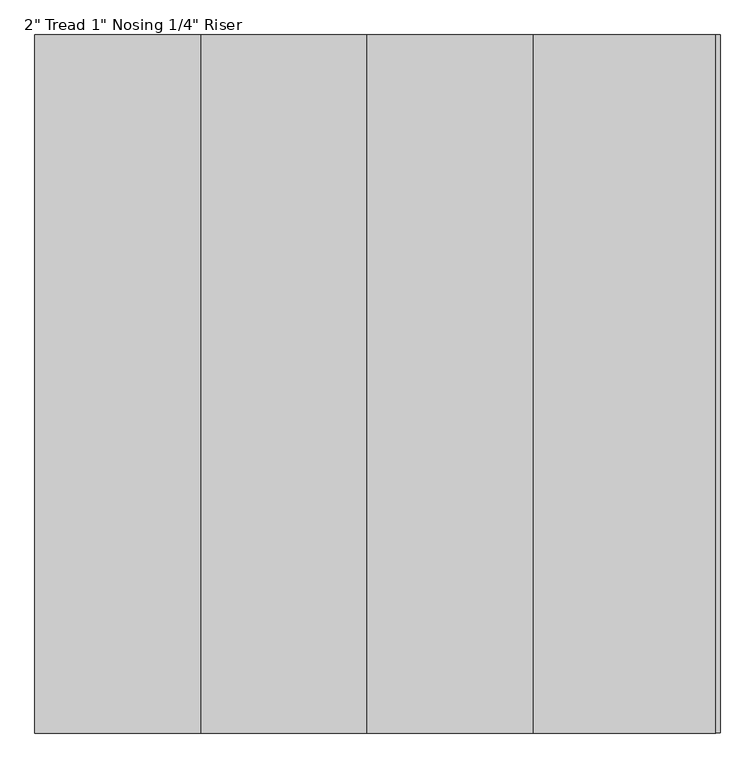
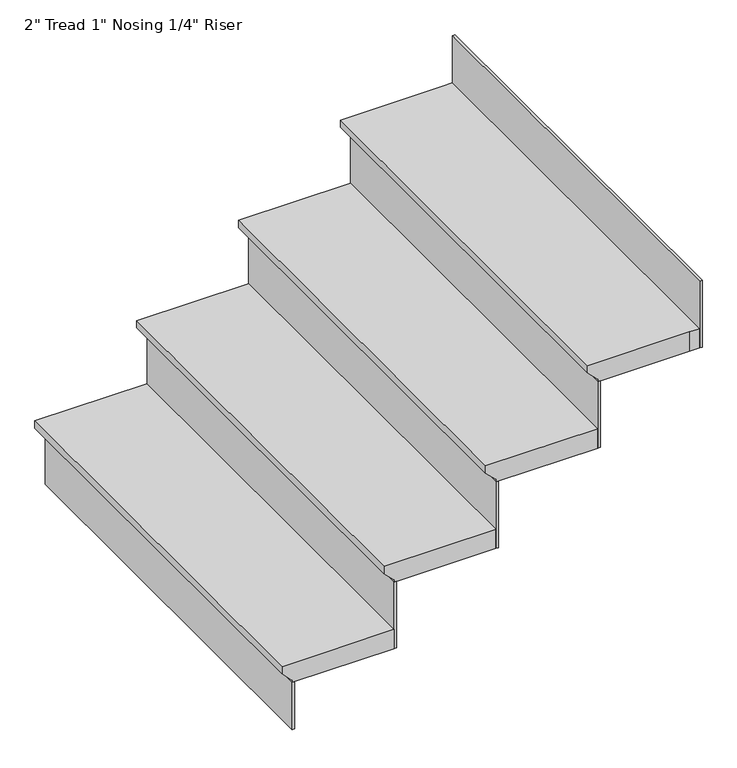
"""IFC4 building model written with IfcOpenShell, lengths in millimetres: stair flight geometry."""

from ifc_helpers import new_model, si_unit, origin, place, context, project, spatial, faceted_brep, source, transform, mapped, element, save


def stair_flight_49469ed7(model_context):
    return source(origin(), model_context, "Body", "Brep", [
        faceted_brep([(16662.7916032, 5155.1241878, 156.21), (16662.7916032, 5155.1241878, 175.26), (16662.7916032, 6221.9241878, 175.26), (16662.7916032, 6221.9241878, 156.21), (16688.1916032, 5155.1241878, 130.81), (16688.1916032, 6221.9241878, 130.81), (16942.1916032, 5155.1241878, 175.26), (16942.1916032, 6221.9241878, 175.26), (16688.1916032, 6221.9241878, 124.46), (16942.1916032, 6221.9241878, 124.46), (16942.1916032, 5155.1241878, 124.46), (16688.1916032, 5155.1241878, 124.46)], [[[0, 1, 2, 3]], [[4, 0, 3, 5]], [[2, 1, 6, 7]], [[8, 9, 10, 11]], [[2, 7, 9, 8, 5, 3]], [[8, 11, 4, 5]], [[6, 1, 0, 4, 11, 10]], [[7, 6, 10, 9]]]),
        faceted_brep([(16688.1916032, 5155.1241878, 124.46), (16688.1916032, 5155.1241878, 0.0), (16694.5416032, 5155.1241878, 0.0), (16694.5416032, 5155.1241878, 124.46), (16688.1916032, 6221.9241878, 124.46), (16694.5416032, 6221.9241878, 124.46), (16694.5416032, 6221.9241878, 0.0), (16688.1916032, 6221.9241878, 0.0)], [[[0, 1, 2, 3]], [[4, 5, 6, 7]], [[1, 0, 4, 7]], [[2, 1, 7, 6]], [[3, 2, 6, 5]], [[0, 3, 5, 4]]]),
        faceted_brep([(16942.1916032, 5155.1241878, 299.72), (16942.1916032, 5155.1241878, 124.46), (16948.5416032, 5155.1241878, 124.46), (16948.5416032, 5155.1241878, 299.72), (16942.1916032, 6221.9241878, 299.72), (16948.5416032, 6221.9241878, 299.72), (16948.5416032, 6221.9241878, 124.46), (16942.1916032, 6221.9241878, 124.46)], [[[0, 1, 2, 3]], [[4, 5, 6, 7]], [[1, 0, 4, 7]], [[2, 1, 7, 6]], [[3, 2, 6, 5]], [[0, 3, 5, 4]]]),
        faceted_brep([(16916.7916032, 6221.9241878, 350.52), (16916.7916032, 5155.1241878, 350.52), (17196.1916032, 5155.1241878, 350.52), (17196.1916032, 6221.9241878, 350.52), (16942.1916032, 6221.9241878, 299.72), (17196.1916032, 6221.9241878, 299.72), (17196.1916032, 5155.1241878, 299.72), (16942.1916032, 5155.1241878, 299.72), (16942.1916032, 6221.9241878, 306.07), (16916.7916032, 6221.9241878, 331.47), (16942.1916032, 5155.1241878, 306.07), (16916.7916032, 5155.1241878, 331.47)], [[[0, 1, 2, 3]], [[4, 5, 6, 7]], [[0, 3, 5, 4, 8, 9]], [[4, 7, 10, 8]], [[2, 1, 11, 10, 7, 6]], [[3, 2, 6, 5]], [[11, 1, 0, 9]], [[10, 11, 9, 8]]]),
        faceted_brep([(17196.1916032, 5155.1241878, 474.98), (17196.1916032, 5155.1241878, 299.72), (17202.5416032, 5155.1241878, 299.72), (17202.5416032, 5155.1241878, 474.98), (17196.1916032, 6221.9241878, 474.98), (17202.5416032, 6221.9241878, 474.98), (17202.5416032, 6221.9241878, 299.72), (17196.1916032, 6221.9241878, 299.72)], [[[0, 1, 2, 3]], [[4, 5, 6, 7]], [[1, 0, 4, 7]], [[2, 1, 7, 6]], [[3, 2, 6, 5]], [[0, 3, 5, 4]]]),
        faceted_brep([(17170.7916032, 6221.9241878, 525.78), (17170.7916032, 5155.1241878, 525.78), (17450.1916032, 5155.1241878, 525.78), (17450.1916032, 6221.9241878, 525.78), (17196.1916032, 6221.9241878, 474.98), (17450.1916032, 6221.9241878, 474.98), (17450.1916032, 5155.1241878, 474.98), (17196.1916032, 5155.1241878, 474.98), (17196.1916032, 6221.9241878, 481.33), (17170.7916032, 6221.9241878, 506.73), (17196.1916032, 5155.1241878, 481.33), (17170.7916032, 5155.1241878, 506.73)], [[[0, 1, 2, 3]], [[4, 5, 6, 7]], [[0, 3, 5, 4, 8, 9]], [[4, 7, 10, 8]], [[2, 1, 11, 10, 7, 6]], [[3, 2, 6, 5]], [[11, 1, 0, 9]], [[10, 11, 9, 8]]]),
        faceted_brep([(17704.1916032, 5155.1241878, 825.5), (17704.1916032, 5155.1241878, 650.24), (17710.5416032, 5155.1241878, 650.24), (17710.5416032, 5155.1241878, 825.5), (17704.1916032, 6221.9241878, 825.5), (17710.5416032, 6221.9241878, 825.5), (17710.5416032, 6221.9241878, 650.24), (17704.1916032, 6221.9241878, 650.24)], [[[0, 1, 2, 3]], [[4, 5, 6, 7]], [[1, 0, 4, 7]], [[2, 1, 7, 6]], [[3, 2, 6, 5]], [[0, 3, 5, 4]]]),
        faceted_brep([(17450.1916032, 5155.1241878, 650.24), (17450.1916032, 5155.1241878, 474.98), (17456.5416032, 5155.1241878, 474.98), (17456.5416032, 5155.1241878, 650.24), (17450.1916032, 6221.9241878, 650.24), (17456.5416032, 6221.9241878, 650.24), (17456.5416032, 6221.9241878, 474.98), (17450.1916032, 6221.9241878, 474.98)], [[[0, 1, 2, 3]], [[4, 5, 6, 7]], [[1, 0, 4, 7]], [[2, 1, 7, 6]], [[3, 2, 6, 5]], [[0, 3, 5, 4]]]),
        faceted_brep([(17704.1916032, 6221.9241878, 701.04), (17678.7916032, 6221.9241878, 701.04), (17424.7916032, 6221.9241878, 701.04), (17424.7916032, 5155.1241878, 701.04), (17678.7916032, 5155.1241878, 701.04), (17704.1916032, 5155.1241878, 701.04), (17678.7916032, 6221.9241878, 650.24), (17704.1916032, 6221.9241878, 650.24), (17704.1916032, 5155.1241878, 650.24), (17678.7916032, 5155.1241878, 650.24), (17450.1916032, 5155.1241878, 650.24), (17450.1916032, 6221.9241878, 650.24), (17450.1916032, 6221.9241878, 656.59), (17424.7916032, 6221.9241878, 681.99), (17450.1916032, 5155.1241878, 656.59), (17424.7916032, 5155.1241878, 681.99)], [[[0, 1, 2, 3, 4, 5]], [[6, 7, 8, 9, 10, 11]], [[1, 0, 7, 6]], [[2, 1, 6, 11, 12, 13]], [[11, 10, 14, 12]], [[4, 3, 15, 14, 10, 9]], [[5, 4, 9, 8]], [[0, 5, 8, 7]], [[15, 3, 2, 13]], [[14, 15, 13, 12]]]),
    ])


if __name__ == "__main__":
    model = new_model("IFC4")
    model_context = context("Model", 3, world=origin())
    ifc_project = project(units=[si_unit("LENGTHUNIT", "METRE", prefix="MILLI")], contexts=[model_context])
    site = spatial("IfcSite", under=ifc_project)
    building = spatial("IfcBuilding", under=site)
    placement = place(None, origin())
    stair_flight_shape = stair_flight_49469ed7(model_context)
    element("IfcStairFlight", 1, ObjectType="2\" Tread 1\" Nosing 1/4\" Riser", at=placement, inside=building, context=model_context, shape_type="MappedRepresentation", body=[
        mapped(stair_flight_shape, transform((0.0, 0.0, 0.0), x_axis=(1.0, 0.0, 0.0), y_axis=(0.0, 1.0, 0.0), z_axis=(0.0, 0.0, 1.0))),
    ])
    save(model, "model.ifc")
